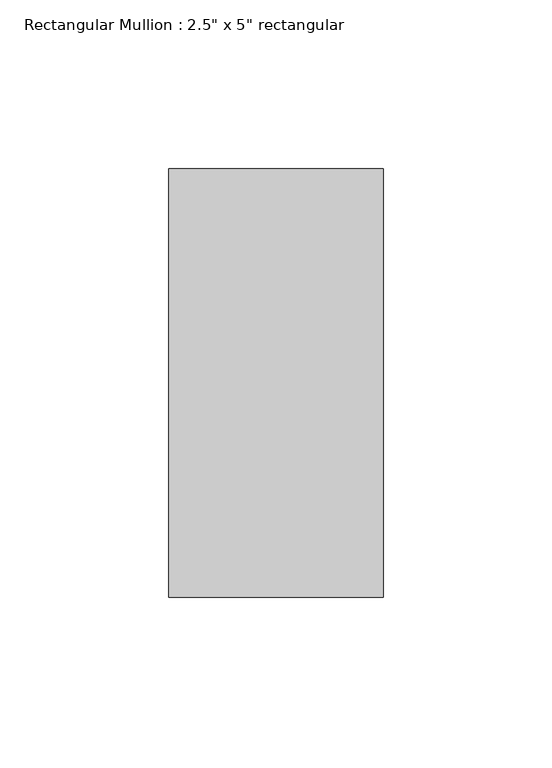
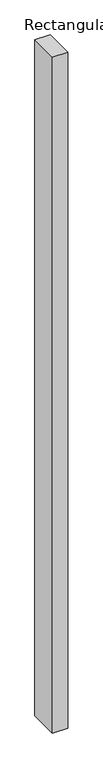
"""IFC4 building model written with IfcOpenShell, lengths in millimetres: member geometry."""

from ifc_helpers import new_model, si_unit, frame, origin, place, context, project, spatial, polyline, outline, extrude, source, transform, mapped, element, save


def member_db480205(model_context):
    return source(origin(), model_context, "Body", "SweptSolid", [
        extrude(outline(polyline([(0.0, 63.5), (0.0, -63.5), (-63.5, -63.5), (-63.5, 63.5), (0.0, 63.5)])), frame((0.0, 0.0, -2984.5), z_axis=(0.0, 0.0, 1.0), x_axis=(1.0, 0.0, 0.0)), (0.0, 0.0, 1.0), 2984.5),
    ])


if __name__ == "__main__":
    model = new_model("IFC4")
    model_context = context("Model", 3, world=origin())
    ifc_project = project(units=[si_unit("LENGTHUNIT", "METRE", prefix="MILLI")], contexts=[model_context])
    site = spatial("IfcSite", under=ifc_project)
    building = spatial("IfcBuilding", under=site)
    placement = place(None, origin())
    member_shape = member_db480205(model_context)
    element("IfcMember", 1, ObjectType="Rectangular Mullion : 2.5\" x 5\" rectangular", at=placement, inside=building, context=model_context, shape_type="MappedRepresentation", body=[
        mapped(member_shape, transform((0.0, 0.0, 0.0), x_axis=(1.0, 0.0, 0.0), y_axis=(0.0, 1.0, 0.0), z_axis=(0.0, 0.0, 1.0))),
    ])
    save(model, "model.ifc")

# Revit data of these elements
# Type "Rectangular Mullion : 2.5\" x 5\" rectangular"
#   built-in parameter 1007304 = 0.416667 (stored number, unit not read)
#   built-in parameter 1007301 = 0.104167 (stored number, unit not read)
#   built-in parameter 1007300 = 0.104167 (stored number, unit not read)
# Element 1 (IfcMember, "Rectangular Mullion : 2.5\" x 5\" rectangular")
#   Materials on its faces: "Aluminum"
# Materials
#   "Aluminum": class "Metal", colour RGB 247 247 247, transparency 0, Description = "Aluminum 6061", Cost = 0
